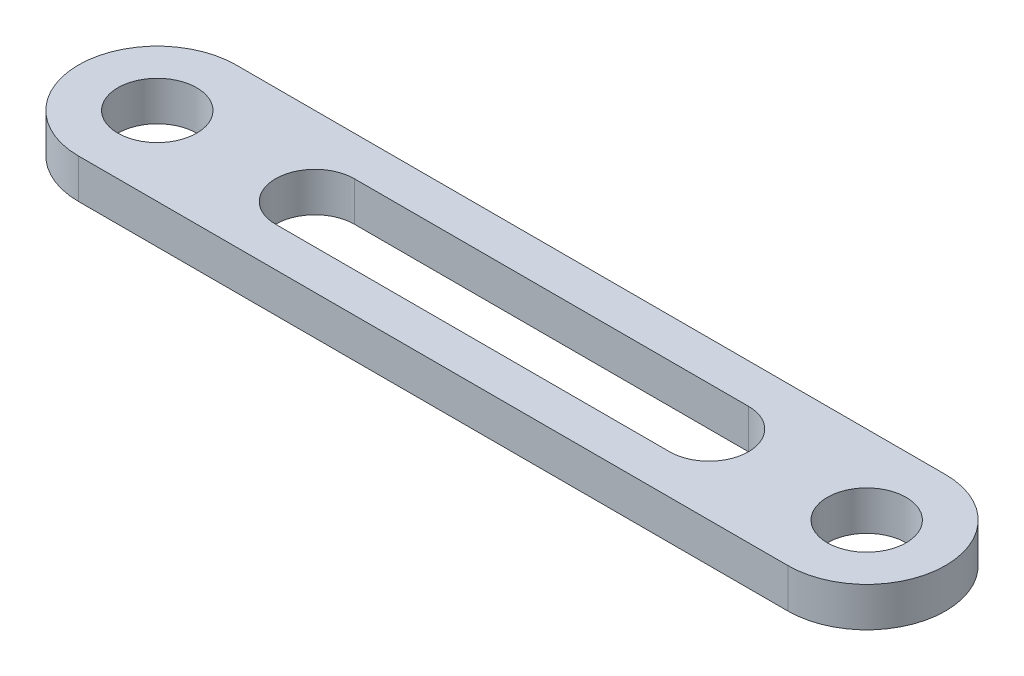
from build123d import *

# Parameters (mm, degrees)
LINK_PROFILE_SKETCH_R = 5
LINK_PLATE_5MM_DEPTH  = 5


with BuildPart() as part:
    # Link Profile Sketch → Link Plate 5mm (new body)
    with BuildSketch(Plane(origin=(0, 0, 0), x_dir=(1, 0, 0), z_dir=(0, 1, 0))):
        with BuildLine():
            Line((-45, 10), (45, 10))
            ThreePointArc((45, 10), (55, 0), (45, -10))
            Line((45, -10), (-45, -10))
            ThreePointArc((-45, -10), (-55, 0), (-45, 10))
        make_face()
        with Locations(Location((-45, 0, 0), (0, 0, 270))):
            Circle(LINK_PROFILE_SKETCH_R, mode=Mode.SUBTRACT)
        with Locations(Location((45, 0, 0), (0, 0, 270))):
            Circle(LINK_PROFILE_SKETCH_R, mode=Mode.SUBTRACT)
        with BuildLine():
            Line((-25, 5), (25, 5))
            ThreePointArc((25, 5), (30, 0), (25, -5))
            Line((25, -5), (-25, -5))
            ThreePointArc((-25, -5), (-30, 0), (-25, 5))
        make_face(mode=Mode.SUBTRACT)
    extrude(amount=LINK_PLATE_5MM_DEPTH)


solid = part.part
